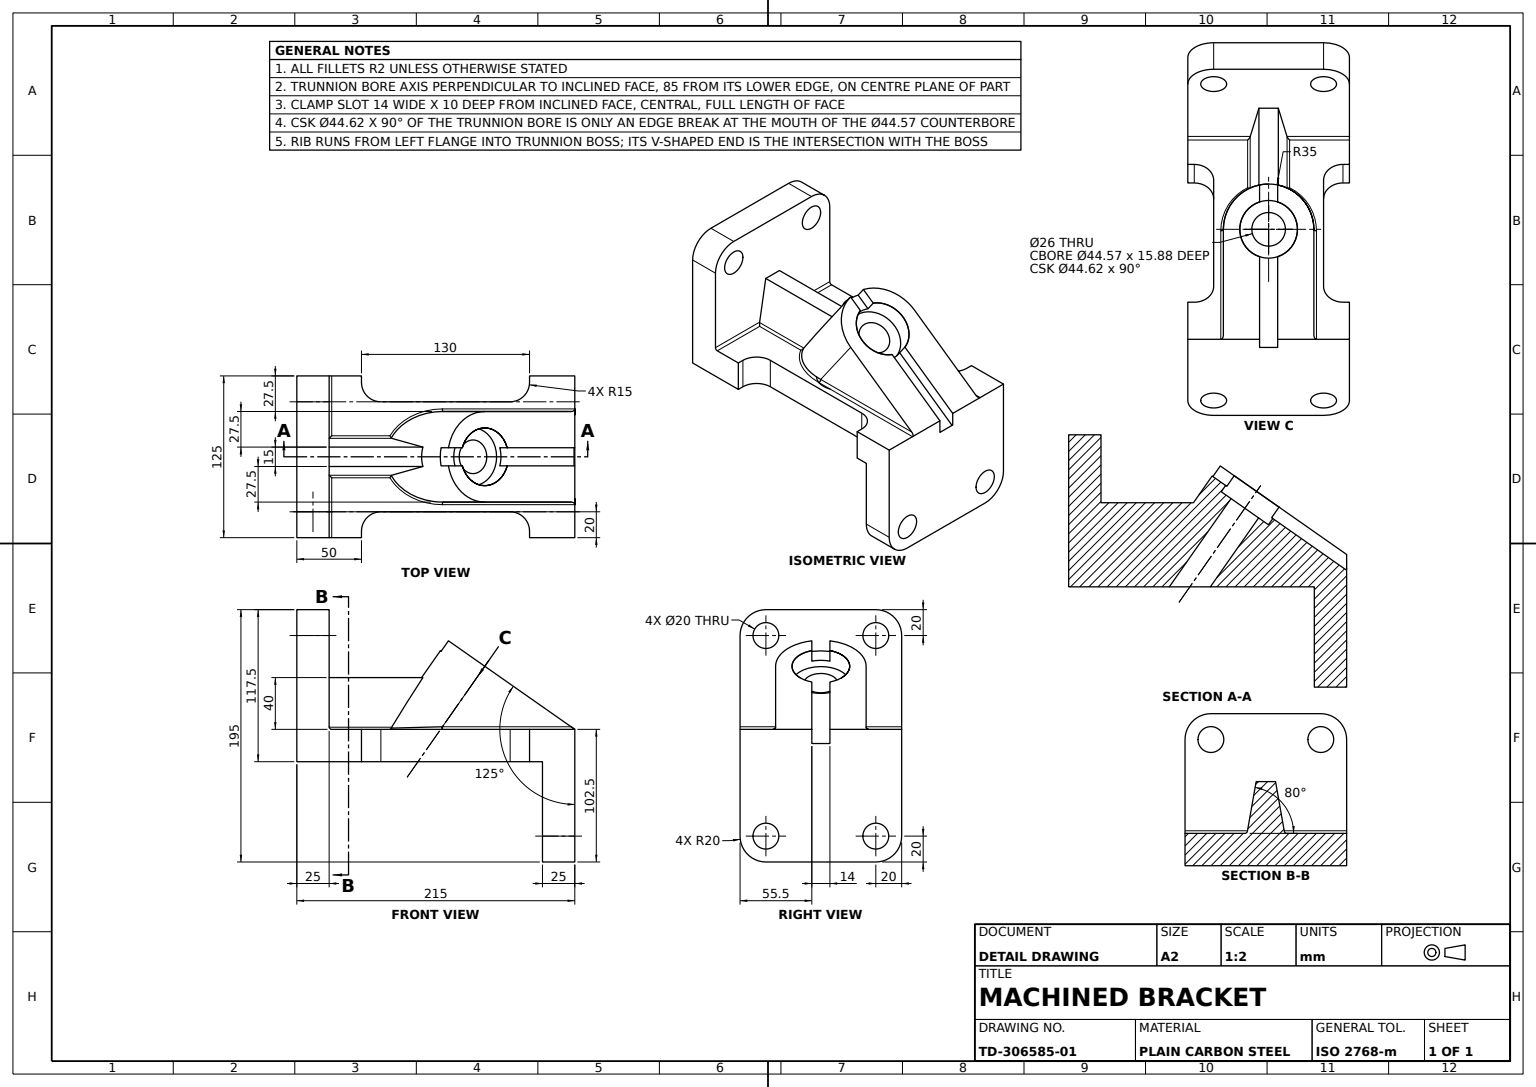
from build123d import *

# Parameters (mm, degrees)
BASE_PLATE_DEPTH             = 25
END_FLANGE_A_SKETCH_R        = 10
END_FLANGE_A_DEPTH           = 25
END_FLANGE_B_SKETCH_R        = 10
END_FLANGE_B_DEPTH           = 25
ANGLED_TRUNNION_BOSS_REACH   = 222.848
CLAMP_SLOT_SKETCH_W          = 135
CLAMP_SLOT_SKETCH_H          = 14
CLAMP_SLOT_14MM_DEPTH        = 10
SUPPORT_RIB_15MM_REACH       = 173.081
SUPPORT_RIB_SKETCH_WALL_W    = 415.677593096
SUPPORT_RIB_SKETCH_WALL_H    = 15
SUPPORT_RIB_15MM_DRAFT_ANGLE = 10
EDGE_FILLETS_R2_R            = 2


with BuildPart() as part:
    # Base Plate Sketch → Base Plate (new body)
    with BuildSketch(Plane(origin=(0, 0, 0), x_dir=(1, 0, 0), z_dir=(0, 1, 0))):
        with BuildLine():
            Line((72.5, 62.5), (107.5, 62.5))
            Line((107.5, 62.5), (107.5, -62.5))
            Line((107.5, -62.5), (72.5, -62.5))
            Line((72.5, -62.5), (72.5, -57.5))
            ThreePointArc((72.5, -57.5), (68.106601718, -46.893398282), (57.5, -42.5))
            Line((57.5, -42.5), (-42.5, -42.5))
            ThreePointArc((-42.5, -42.5), (-53.106601718, -46.893398282), (-57.5, -57.5))
            Line((-57.5, -57.5), (-57.5, -62.5))
            Line((-57.5, -62.5), (-107.5, -62.5))
            Line((-107.5, -62.5), (-107.5, 62.5))
            Line((-107.5, 62.5), (-57.5, 62.5))
            Line((-57.5, 62.5), (-57.5, 57.5))
            ThreePointArc((-57.5, 57.5), (-53.106601718, 46.893398282), (-42.5, 42.5))
            Line((-42.5, 42.5), (57.5, 42.5))
            ThreePointArc((57.5, 42.5), (68.106601718, 46.893398282), (72.5, 57.5))
            Line((72.5, 57.5), (72.5, 62.5))
        make_face()
    extrude(amount=BASE_PLATE_DEPTH)

    # End Flange A Sketch → End Flange A (add)
    with BuildSketch(Plane(origin=(107.5, 0, 0), x_dir=(0, 0, -1), z_dir=(1, 0, 0))):
        with BuildLine():
            Line((-62.5, 25), (62.5, 25))
            Line((62.5, 25), (62.5, -57.5))
            ThreePointArc((62.5, -57.5), (56.642135624, -71.642135624), (42.5, -77.5))
            Line((42.5, -77.5), (-42.5, -77.5))
            ThreePointArc((-42.5, -77.5), (-56.642135624, -71.642135624), (-62.5, -57.5))
            Line((-62.5, -57.5), (-62.5, 25))
        make_face()
        with Locations((-42.5, -57.5)):
            Circle(END_FLANGE_A_SKETCH_R, mode=Mode.SUBTRACT)
        with Locations((42.5, -57.5)):
            Circle(END_FLANGE_A_SKETCH_R, mode=Mode.SUBTRACT)
    extrude(amount=-END_FLANGE_A_DEPTH)

    # End Flange B Sketch → End Flange B (add)
    with BuildSketch(Plane.ZY.offset(107.5)):
        with BuildLine():
            Line((-62.5, 0), (62.5, 0))
            Line((62.5, 0), (62.5, 97.5))
            ThreePointArc((62.5, 97.5), (56.642135624, 111.642135624), (42.5, 117.5))
            Line((42.5, 117.5), (-42.5, 117.5))
            ThreePointArc((-42.5, 117.5), (-56.642135624, 111.642135624), (-62.5, 97.5))
            Line((-62.5, 97.5), (-62.5, 0))
        make_face()
        with Locations((-42.5, 97.5)):
            Circle(END_FLANGE_B_SKETCH_R, mode=Mode.SUBTRACT)
        with Locations((42.5, 97.5)):
            Circle(END_FLANGE_B_SKETCH_R, mode=Mode.SUBTRACT)
    extrude(amount=-END_FLANGE_B_DEPTH)

    # Angled Trunnion Boss: up to this face of the body (flat: up to its plane)
    angled_trunnion_boss_end = Plane(part.part.faces().sort_by_distance((13.835650778, 25, 0))[0])
    # Trunnion Boss Sketch → Angled Trunnion Boss (add, up to the picked face)
    with BuildSketch(Plane(origin=(47.112575056, 67.283730159, 0), x_dir=(0, 0, -1), z_dir=(-0.5735764363510502, -0.8191520442889889, 0)), mode=Mode.PRIVATE) as angled_trunnion_boss_sk1:
        with BuildLine():
            Line((-35, -11.280566148), (-35, 73.719433852))
            Line((-35, 73.719433852), (35, 73.719433852))
            Line((35, 73.719433852), (35, -11.280566148))
            ThreePointArc((35, -11.280566148), (0, -46.280566148), (-35, -11.280566148))
        make_face()
    angled_trunnion_boss_tool1 = split(extrude(angled_trunnion_boss_sk1.sketch, amount=ANGLED_TRUNNION_BOSS_REACH, mode=Mode.PRIVATE), bisect_by=angled_trunnion_boss_end, keep=Keep.BOTH, mode=Mode.PRIVATE)
    add(angled_trunnion_boss_tool1.solids().sort_by(Axis((61.205035, 57.416084, 0), (-0.5735764363510502, -0.8191520442889889, 0)))[0])

    # Sketch6 → Trunnion Bore CBORE M24 (revolve, cut)
    with BuildSketch(Plane(origin=(37.872076235, 73.75399709, 0), x_dir=(-0.8191520442889889, 0.5735764363510502, 0), z_dir=(0, 0, 1))):
        Polygon((0, 0), (0, 207.282018355), (13, 207.282018355), (13, 15.9), (22.285, 15.9), (22.285, 0.025), (22.31, 0), align=None)
    revolve(axis=Axis((41.514286606, 78.955612571, 0), (-0.5735764363510502, -0.8191520442889889, 0)), mode=Mode.SUBTRACT)

    # Clamp Slot Sketch → Clamp Slot 14mm (cut)
    with BuildSketch(Plane(origin=(47.112575056, 67.283730159, 0), x_dir=(0.819152044288989, -0.5735764363510502, 0), z_dir=(0.5735764363510502, 0.819152044288989, 0))):
        with Locations((12.5, 0)):
            Rectangle(CLAMP_SLOT_SKETCH_W, CLAMP_SLOT_SKETCH_H)
    extrude(amount=-CLAMP_SLOT_14MM_DEPTH, mode=Mode.SUBTRACT)

    # Support Rib Sketch wall → Support Rib 15mm (add, up to next)
    with BuildSketch(Plane(origin=(-46.742324561, 65, 0), x_dir=(1, 0, 0), z_dir=(0, 1, 0)), mode=Mode.PRIVATE) as support_rib_15mm_sk1:
        Rectangle(SUPPORT_RIB_SKETCH_WALL_W, SUPPORT_RIB_SKETCH_WALL_H)
    support_rib_15mm_tool1 = extrude(support_rib_15mm_sk1.sketch, amount=-SUPPORT_RIB_15MM_REACH, mode=Mode.PRIVATE) - part.part
    add(support_rib_15mm_tool1.solids().sort_by_distance((-46.742324561, 65, 0))[0])

    # Support Rib 15mm draft
    support_rib_15mm_draft_faces = [part.faces().sort_by_distance(p)[0] for p in [
        (-46.742324561, 64.5, -7.5),
        (-46.742324561, 64.5, 7.5),
    ]]
    draft(support_rib_15mm_draft_faces, Plane(origin=(-46.742324561, 65, 0), x_dir=(1, 0, 0), z_dir=(0, 1, 0)), SUPPORT_RIB_15MM_DRAFT_ANGLE)

    # Edge Fillets R2
    edge_fillets_r2_edges = [part.edges().sort_by_distance(p)[0] for p in [
        (55.617079978, 25, 35),
        (55.617079978, 25, -35),
        (-18.472856997, 25, -29.901342917),
        (-18.472856997, 25, 29.901342917),
        (-82.5, 25, -38.526539614),
        (-58.812113156, 25, -14.553079228),
        (-58.812113156, 25, 14.553079228),
        (-82.5, 25, 38.526539614),
    ]]
    fillet(edge_fillets_r2_edges, radius=EDGE_FILLETS_R2_R)


solid = part.part
